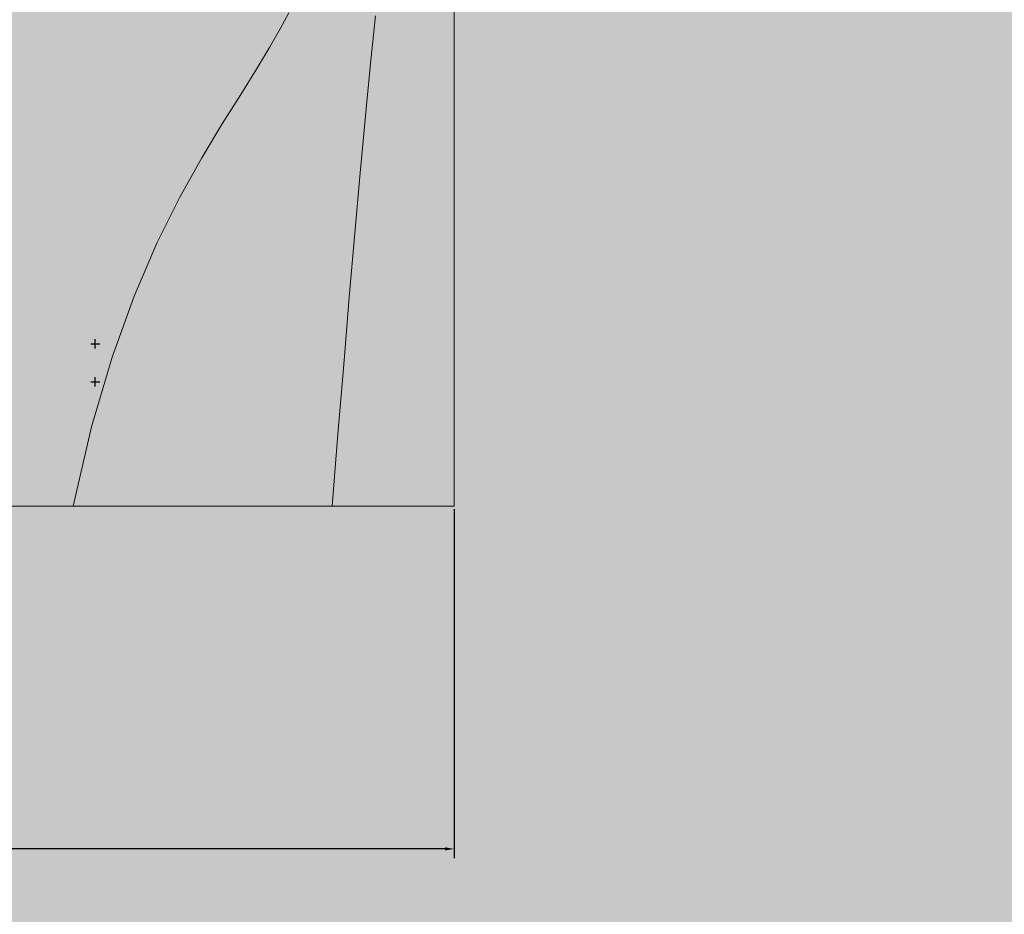
# Model space of a CAD drawing. Units: inches. Extents: x 3024 to 3952, y 1308 to 1863.
# Tile 16 of 29: x 3411.08 to 3430.42, y 1488.75 to 1506.34. Entities that reach past the tile are written whole.
import ezdxf

# ---------------------------------------------------------------- set-up
doc = ezdxf.new("R2010")
doc.units = ezdxf.units.IN
for name, color, linetype, lineweight in [('A-ANNO-DIMS', 2, 'Continuous', 18), ('A-FLOR-TILE-PATT', 7, 'Continuous', 13), ('A-FURN', 8, 'Continuous', 18), ('A-FURN-PATT', 9, 'Continuous', 13)]:
    doc.layers.add(name, color=color, linetype=linetype, lineweight=lineweight)
doc.layers.add('A-FLOR-PATT', color=254, linetype='Continuous', lineweight=13, true_color=0xfeeab9)
doc.styles.get("Standard").update_dxf_attribs({"font": 'arial.ttf'})
doc.dimstyles.get("Standard").update_dxf_attribs({"dimtxt": 0.18, "dimasz": 0.18, "dimexe": 0.18, "dimexo": 0.0625, "dimgap": 0.09, "dimtad": 0, "dimtih": 1, "dimtoh": 1, "dimdec": 4, "dimzin": 0, "dimdsep": 46, "dimtxsty": 'Standard', "dimcen": 0.09, "dimadec": 0, "dimazin": 0, "dimtfac": 1, "dimtdec": 4, "dimtofl": 0, "dimtmove": 0, "dimatfit": 3, "dimfxl": 1, "dimtolj": 1, "dimtzin": 0, "dimarcsym": 0})

# ---------------------------------------------------------------- blocks, each defined once
blk = doc.blocks.new('Table - Rectangular Woodgrain 60 x 30 in.')
for p, q in [((60, 0), (0, 0)), ((60, -30), (60, 0))]:
    blk.add_line(p, q)
for points in [[(47.1333, -2.0667), (48.3862, -2.1947), (49.7625, -2.3281), (51.2513, -2.4663), (52.8416, -2.6083), (54.5226, -2.7535), (56.2833, -2.9011), (58.1127, -3.0501), (60, -3.2)], [(47.0542, -4.3417), (47.4756, -4.5629), (47.9661, -4.8427), (48.5372, -5.1866), (49.2, -5.6), (49.9676, -6.0844), (50.8594, -6.625), (51.8965, -7.2031), (53.1, -7.8), (54.491, -8.3969), (56.0906, -8.975), (57.9199, -9.5156), (60, -10)]]:
    blk.add_lwpolyline(points)
blk = doc.blocks.new('*D33')
at = {"layer": 'A-ANNO-DIMS', "color": 0, "lineweight": -2, "transparency": 16777216}
for p, q in [((3397.15, 1496.716), (3397.15, 1489.858)), ((3419.618, 1496.716), (3419.618, 1489.858)), ((3397.33, 1490.038), (3408.165, 1490.038)), ((3419.438, 1490.038), (3408.604, 1490.038))]:
    blk.add_line(p, q, dxfattribs=at)
at = {"layer": 'A-ANNO-DIMS', "color": 0, "transparency": 16777216}
for points in [[(3397.33, 1490.068), (3397.33, 1490.008), (3397.15, 1490.038)], [(3419.438, 1490.068), (3419.438, 1490.008), (3419.618, 1490.038)]]:
    blk.add_solid(points, dxfattribs=at)
at = {"layer": 'Defpoints', "color": 0, "transparency": 16777216}
for p in [(3397.15, 1496.778), (3419.618, 1496.778), (3419.618, 1490.038)]:
    blk.add_point(p, dxfattribs=at)
at = {"layer": 'A-ANNO-DIMS', "color": 0, "transparency": 16777216, "insert": (3408.384, 1490.038), "char_height": 0.18, "attachment_point": 5}
blk.add_mtext('\\A1;22', dxfattribs=at)
blk = doc.blocks.new('*D107')
at = {"layer": 'A-ANNO-DIMS', "color": 0, "lineweight": -2, "transparency": 16777216}
for p, q in [((3412.475, 1499.22), (3412.655, 1499.22)), ((3412.565, 1499.13), (3412.565, 1499.31)), ((3412.565, 1435.781), (3412.565, 1459.391)), ((3412.745, 1435.781), (3412.565, 1435.781))]:
    blk.add_line(p, q, dxfattribs=at)
at = {"layer": 'A-ANNO-DIMS', "color": 0, "transparency": 16777216}
blk.add_solid([(3412.595, 1459.391), (3412.535, 1459.391), (3412.565, 1459.571)], dxfattribs=at)
at = {"layer": 'Defpoints', "color": 0, "transparency": 16777216}
for p in [(3412.565, 1499.22), (3412.565, 1459.571)]:
    blk.add_point(p, dxfattribs=at)
at = {"layer": 'A-ANNO-DIMS', "color": 0, "transparency": 16777216, "insert": (3413.226, 1435.781), "char_height": 0.18, "attachment_point": 5}
blk.add_mtext('\\A1;R39.65', dxfattribs=at)
blk = doc.blocks.new('*D108')
at = {"layer": 'A-ANNO-DIMS', "color": 0, "lineweight": -2, "transparency": 16777216}
for p, q in [((3412.475, 1499.966), (3412.655, 1499.966)), ((3412.565, 1499.876), (3412.565, 1500.056)), ((3412.565, 1441.651), (3412.565, 1463.339)), ((3412.745, 1441.651), (3412.565, 1441.651))]:
    blk.add_line(p, q, dxfattribs=at)
at = {"layer": 'A-ANNO-DIMS', "color": 0, "transparency": 16777216}
blk.add_solid([(3412.595, 1463.339), (3412.535, 1463.339), (3412.565, 1463.519)], dxfattribs=at)
at = {"layer": 'Defpoints', "color": 0, "transparency": 16777216}
for p in [(3412.565, 1499.966), (3412.565, 1463.519)]:
    blk.add_point(p, dxfattribs=at)
at = {"layer": 'A-ANNO-DIMS', "color": 0, "transparency": 16777216, "insert": (3413.226, 1441.651), "char_height": 0.18, "attachment_point": 5}
blk.add_mtext('\\A1;R36.45', dxfattribs=at)

msp = doc.modelspace()

# ---------------------------------------------------------------- hatches: boundary and pattern name
at = {"layer": 'A-FLOR-PATT', "transparency": 33554528}
h = msp.add_hatch(color=256, dxfattribs=at)
h.dxf.hatch_style = 1
h.paths.add_polyline_path([(3460.764, 1688.6064), (3412.764, 1688.6064), (3412.764, 1694.6064), (3460.764, 1694.6064), (3460.764, 1778.6064), (3406.764, 1778.6064), (3406.764, 1759.9514), (3318.2981, 1759.9514), (3318.2981, 1658.6064), (3322.5356, 1658.6064), (3322.5356, 1652.6064), (3292.764, 1652.6064), (3292.764, 1778.6064), (3106.764, 1778.6064), (3106.764, 1628.6064), (3172.764, 1628.6064), (3172.764, 1532.6064), (3166.764, 1532.6064), (3166.764, 1628.6064), (3106.764, 1628.6064), (3106.764, 1356.8452), (3202.812, 1356.8452), (3202.812, 1354.2534), (3202.812, 1353.8388), (3202.812, 1351.1212), (3202.812, 1347.8452), (3277.764, 1347.8452), (3277.764, 1353.8452), (3277.764, 1356.8452), (3277.764, 1442.6064), (3460.764, 1442.6064)])
h.paths.add_polyline_path([(3216.238, 1527.2064), (3216.238, 1491.2064), (3214.663, 1491.2064), (3214.663, 1491.2409, -0.3966224), (3180.243, 1526.6064), (3163.0285, 1526.6064), (3163.0285, 1531.1064), (3161.716, 1531.1064), (3161.716, 1561.1064), (3163.0285, 1561.1064), (3163.0285, 1531.1064), (3163.0285, 1526.6064), (3180.243, 1526.6064, 0.3966224), (3214.663, 1491.2409), (3214.663, 1527.2064)], flags=16)
h.paths.add_polyline_path([(3227.364, 1649.8972), (3191.364, 1649.8972), (3191.364, 1651.4722), (3227.364, 1651.4722)], flags=16)
h.paths.add_polyline_path([(3323.1172, 1606.7362), (3323.8545, 1606.8514), (3323.8545, 1594.8241), (3323.1172, 1594.9393)], flags=16)
h.paths.add_polyline_path([(3324.2232, 1606.909), (3330.1216, 1607.8307), (3330.1216, 1614.1093), (3339.3495, 1614.1093), (3340.2711, 1620.0078), (3352.4136, 1620.0078), (3353.3353, 1614.1093), (3359.9941, 1614.1093), (3360.9157, 1620.0078), (3373.0582, 1620.0078), (3373.9799, 1614.1093), (3383.2077, 1614.1093), (3383.2077, 1607.8307), (3389.1062, 1606.909), (3389.1062, 1594.7665), (3383.2077, 1593.8449), (3383.2077, 1587.5663), (3373.9799, 1587.5663), (3373.0583, 1581.6678), (3360.9157, 1581.6678), (3359.9941, 1587.5663), (3353.3353, 1587.5663), (3352.4136, 1581.6678), (3340.2711, 1581.6678), (3339.3495, 1587.5663), (3330.1216, 1587.5663), (3330.1216, 1593.8449), (3324.2232, 1594.7665)], flags=16)
h.paths.add_polyline_path([(3236.1584, 1693.1064), (3236.1584, 1723.1064), (3237.4709, 1723.1064), (3237.4709, 1693.1064)], flags=16)
h.paths.add_polyline_path([(3373.2158, 1600.6847), (3373.7965, 1600.7303), (3374.3268, 1600.7874), (3374.8132, 1600.8531), (3375.2621, 1600.9247), (3375.6801, 1600.9991), (3376.0736, 1601.0735), (3376.6855, 1601.19), (3377.366, 1601.3023), (3378.0667, 1601.3814), (3378.8026, 1601.4123), (3379.5865, 1601.3839), (3380.4537, 1601.2948), (3381.301, 1601.1717), (3382.0317, 1601.0433), (3382.4398, 1600.9607), (3382.6252, 1600.9201), (3382.919, 1600.8507), (3382.9044, 1600.8531), (3382.842, 1600.8678), (3382.7541, 1600.8896), (3382.6252, 1600.9201), (3382.4398, 1600.9607), (3382.1868, 1601.0119), (3381.8738, 1601.0711), (3381.5125, 1601.1346), (3381.1149, 1601.1988), (3380.6928, 1601.2601), (3380.2581, 1601.3149), (3379.8226, 1601.3597), (3379.3984, 1601.3908), (3378.9944, 1601.4054), (3378.6092, 1601.4042), (3378.2384, 1601.3886), (3377.8777, 1601.36), (3377.5227, 1601.32), (3377.1691, 1601.2698), (3376.8127, 1601.211), (3376.4491, 1601.145), (3376.0736, 1601.0735), (3375.4177, 1600.9494), (3374.5542, 1600.8119), (3373.5044, 1600.6988)], flags=0)
h.paths.add_polyline_path([(3380.0253, 1596.7351), (3380.499, 1596.6659), (3380.9706, 1596.6119), (3381.4375, 1596.5791), (3381.8971, 1596.5736), (3382.5886, 1596.6167), (3382.7848, 1596.6692), (3382.1465, 1596.5706), (3381.236, 1596.5815), (3380.3199, 1596.6865)], flags=0)
h.paths.add_polyline_path([(3369.6414, 1603.9617), (3370.1589, 1604.0021), (3370.6218, 1604.0539), (3371.0335, 1604.1173), (3371.3978, 1604.1921), (3371.7181, 1604.2785), (3371.9984, 1604.3761), (3372.2441, 1604.483), (3372.4611, 1604.5972), (3372.655, 1604.7163), (3372.8317, 1604.8384), (3372.9968, 1604.9611), (3373.3703, 1605.2455), (3373.8426, 1605.5328), (3374.4624, 1605.7539), (3375.1058, 1605.8302), (3375.7221, 1605.8261), (3376.4109, 1605.76), (3377.1534, 1605.6376), (3377.8945, 1605.473), (3378.1382, 1605.409), (3377.7394, 1605.5074), (3377.3509, 1605.5937), (3376.9704, 1605.6677), (3376.5999, 1605.7288), (3376.2417, 1605.7762), (3375.8979, 1605.8092), (3375.5707, 1605.8271), (3375.2621, 1605.8291), (3374.9745, 1605.8146), (3374.7092, 1605.7832), (3374.4647, 1605.7359), (3374.239, 1605.6742), (3374.0298, 1605.5996), (3373.835, 1605.5134), (3373.6525, 1605.4171), (3373.4801, 1605.3123), (3373.3156, 1605.2002), (3373.1562, 1605.0825), (3372.7603, 1604.781), (3372.236, 1604.4588), (3371.5738, 1604.2283), (3370.8493, 1604.0794), (3369.9262, 1603.976)], flags=0)
h.paths.add_polyline_path([(3366.7533, 1606.5832), (3367.1713, 1606.5519), (3367.5378, 1606.5374), (3367.8568, 1606.5394), (3368.1325, 1606.5573), (3368.3694, 1606.5903), (3368.5717, 1606.6377), (3368.7438, 1606.6988), (3368.89, 1606.7728), (3369.0146, 1606.8591), (3369.121, 1606.9568), (3369.2094, 1607.0646), (3369.2792, 1607.181), (3369.3295, 1607.3046), (3369.3596, 1607.4339), (3369.3688, 1607.5676), (3369.3565, 1607.7042), (3369.3218, 1607.8422), (3369.2649, 1607.9804), (3369.1893, 1608.1187), (3369.0993, 1608.2569), (3368.9992, 1608.3952), (3368.8934, 1608.5334), (3368.7861, 1608.6717), (3368.6817, 1608.8099), (3368.4212, 1609.1804), (3368.2685, 1609.7106), (3368.4883, 1610.1814), (3369.0537, 1610.4604), (3369.6717, 1610.5097), (3370.2812, 1610.3612), (3370.4805, 1610.2968), (3370.1882, 1610.3839), (3369.9284, 1610.4472), (3369.6905, 1610.4842), (3369.4662, 1610.4933), (3369.2555, 1610.4765), (3369.0608, 1610.4367), (3368.884, 1610.3767), (3368.7274, 1610.2994), (3368.5931, 1610.2077), (3368.4833, 1610.1045), (3368.4002, 1609.9927), (3368.3451, 1609.8747), (3368.3166, 1609.7517), (3368.3127, 1609.6244), (3368.331, 1609.4935), (3368.3696, 1609.3597), (3368.4261, 1609.2237), (3368.4985, 1609.0863), (3368.5845, 1608.9482), (3368.6817, 1608.8099), (3368.7861, 1608.6717), (3368.8934, 1608.5334), (3368.9992, 1608.3952), (3369.0993, 1608.2569), (3369.3398, 1607.8876), (3369.3941, 1607.2896), (3368.9774, 1606.7817), (3368.3928, 1606.5742), (3367.7162, 1606.5303), (3367.0044, 1606.5585)], flags=0)
h.paths.add_polyline_path([(3362.1859, 1610.2589), (3362.5478, 1610.2845), (3362.8348, 1610.3275), (3363.0585, 1610.3863), (3363.2303, 1610.4595), (3363.3619, 1610.5457), (3363.463, 1610.6432), (3363.5376, 1610.7502), (3363.5876, 1610.8643), (3363.6153, 1610.9834), (3363.6229, 1611.1055), (3363.6125, 1611.2283), (3363.5861, 1611.3496), (3363.5462, 1611.4673), (3363.4949, 1611.5797), (3363.4358, 1611.6871), (3363.3723, 1611.7902), (3363.3081, 1611.8897), (3363.2468, 1611.9863), (3363.192, 1612.0808), (3363.0258, 1612.4261), (3363.3371, 1612.8672), (3363.9008, 1612.9782), (3364.4822, 1612.9641), (3365.1098, 1612.9074), (3365.328, 1612.8805), (3364.9615, 1612.9208), (3364.6426, 1612.9496), (3364.3668, 1612.9669), (3364.1299, 1612.9726), (3363.9276, 1612.9669), (3363.7555, 1612.9496), (3363.6093, 1612.9208), (3363.4848, 1612.8805), (3363.3782, 1612.8289), (3363.2889, 1612.7672), (3363.2169, 1612.6969), (3363.1622, 1612.6193), (3363.1247, 1612.5361), (3363.1046, 1612.4484), (3363.1017, 1612.358), (3363.1161, 1612.266), (3363.1472, 1612.1738), (3363.192, 1612.0808), (3363.2468, 1611.9863), (3363.3081, 1611.8897), (3363.3723, 1611.7902), (3363.4358, 1611.6871), (3363.6363, 1611.323), (3363.5979, 1610.7003), (3363.0863, 1610.3651), (3362.3983, 1610.2622)], flags=0)
h.paths.add_polyline_path([(3352.356, 1581.2991), (3352.2408, 1580.5618), (3340.4439, 1580.5618), (3340.3287, 1581.2991)], flags=16)
h.paths.add_polyline_path([(3340.4439, 1621.1137), (3352.2408, 1621.1137), (3352.356, 1620.3764), (3340.3287, 1620.3764)], flags=16)
h.paths.add_polyline_path([(3278.4282, 1504.7424), (3290.3831, 1504.7424), (3290.3831, 1502.7499), (3291.0473, 1502.7499), (3291.0473, 1494.7799), (3290.3831, 1494.7799), (3290.3831, 1494.1158), (3291.0473, 1494.1158), (3291.0473, 1486.1458), (3290.3831, 1486.1458), (3290.3831, 1484.1533), (3291.0473, 1484.1533), (3291.0473, 1483.4892, -0.0909091), (3291.0473, 1468.8776), (3291.0473, 1468.2135), (3290.3831, 1468.2135), (3290.3831, 1464.8926), (3278.4282, 1464.8926), (3278.4282, 1472.8626), (3277.764, 1473.5268), (3277.764, 1478.84), (3278.4282, 1479.5042)], flags=16)
h.paths.add_polyline_path([(3278.7603, 1504.4103), (3290.051, 1504.4103), (3290.051, 1465.2247), (3278.7603, 1465.2247)], flags=0)
h.paths.add_polyline_path([(3123.904, 1600.7821), (3117.9039, 1602.7821), (3117.9039, 1599.7821), (3119.4039, 1599.7821), (3119.4039, 1596.7821), (3118.4039, 1596.7821), (3118.4039, 1598.7821), (3117.9039, 1598.7821), (3117.9039, 1596.2821), (3109.9039, 1596.2821), (3109.9039, 1617.2821), (3117.9039, 1617.2821), (3117.9039, 1610.7821), (3123.9038, 1612.7821, -0.7025712), (3137.9039, 1606.7822, -0.7025621)], flags=16)
h.paths.add_polyline_path([(3123.9039, 1602.7822), (3123.9039, 1610.7822, -0.7345333), (3136.9039, 1606.7822, -0.7345297)], flags=0)
h.paths.add_polyline_path([(3177.972, 1689.6473), (3109.2405, 1689.6473), (3109.2405, 1741.1959), (3177.972, 1741.1959)], flags=16)
h.paths.add_polyline_path([(3373.0006, 1581.2991), (3372.8854, 1580.5618), (3361.0885, 1580.5618), (3360.9733, 1581.2991)], flags=16)
h.paths.add_polyline_path([(3361.0885, 1621.1137), (3372.8854, 1621.1137), (3373.0006, 1620.3764), (3360.9733, 1620.3764)], flags=16)
h.paths.add_polyline_path([(3116.9039, 1598.2821, -0.4142136), (3116.1539, 1597.2821), (3111.9039, 1597.2821, -0.4142136), (3110.9039, 1598.0321), (3110.9039, 1615.2821, -0.4142136), (3111.6539, 1616.2821), (3115.9039, 1616.2821, -0.4142136), (3116.9039, 1615.5321)], flags=0)
h.paths.add_polyline_path([(3121.6122, 1728.1369), (3121.6122, 1696.5205), (3110.2715, 1696.5205), (3110.2715, 1714.3906), (3121.6122, 1714.3906), (3121.6122, 1716.4526), (3110.2715, 1716.4526), (3110.2715, 1734.3228), (3123.3304, 1734.3228), (3123.3304, 1729.8552), (3134.6711, 1741.1959), (3134.6711, 1728.1369)], flags=0)
h.paths.add_polyline_path([(3389.4748, 1606.8514), (3390.2122, 1606.7362), (3390.2122, 1594.9393), (3389.4748, 1594.8241)], flags=16)
h.paths.add_polyline_path([(3257.6842, 1762.8281), (3259.6842, 1768.8281), (3256.6842, 1768.8281), (3256.6842, 1767.3281), (3253.6842, 1767.3281), (3253.6842, 1768.3281), (3255.6842, 1768.3281), (3255.6842, 1768.8281), (3253.1842, 1768.8281), (3253.1842, 1776.8281), (3274.1842, 1776.8281), (3274.1842, 1768.8281), (3267.6842, 1768.8281), (3269.6842, 1762.8282, -0.7025712), (3263.6843, 1748.8282, -0.7025621)], flags=16)
h.paths.add_polyline_path([(3259.6842, 1762.8281), (3267.6843, 1762.8281, -0.7345333), (3263.6842, 1749.8282, -0.7345297)], flags=0)
h.paths.add_polyline_path([(3411.264, 1715.6064), (3411.264, 1716.9189), (3441.264, 1716.9189), (3441.264, 1715.6064)], flags=16)
h.paths.add_polyline_path([(3178.3806, 1449.1876), (3178.3806, 1397.639), (3109.6491, 1397.639), (3109.6491, 1449.1876)], flags=16)
h.paths.add_polyline_path([(3397.1501, 1541.7146), (3419.6183, 1541.7146), (3419.6183, 1496.7783), (3397.1501, 1496.7783)], flags=16)
h.paths.add_polyline_path([(3254.1842, 1770.5781), (3254.1842, 1774.8281, -0.4142136), (3254.9342, 1775.8281), (3272.1842, 1775.8281, -0.4142136), (3273.1842, 1775.0781), (3273.1842, 1770.8281, -0.4142136), (3272.4342, 1769.8281), (3255.1842, 1769.8281, -0.4142136)], flags=0)
h.paths.add_polyline_path([(3403.672, 1500.7601), (3403.6016, 1500.3997), (3403.5328, 1500.0441), (3403.4662, 1499.6867), (3403.4027, 1499.3226), (3403.3464, 1498.9532), (3403.3025, 1498.5811), (3403.2759, 1498.2091), (3403.2714, 1497.8401), (3403.3064, 1497.2813), (3403.3491, 1497.1219), (3403.2689, 1497.6395), (3403.2778, 1498.3719), (3403.3635, 1499.0984), (3403.4889, 1499.8168), (3403.6016, 1500.3997), (3403.672, 1500.7601), (3403.744, 1501.1315), (3403.817, 1501.5205), (3403.891, 1501.9336), (3403.9656, 1502.3769), (3404.0404, 1502.8572), (3404.115, 1503.3786), (3404.2264, 1504.2311), (3404.2571, 1504.5223), (3404.1552, 1503.6598), (3404.0063, 1502.6193), (3403.8604, 1501.7518), (3403.744, 1501.1315)], flags=0)
h.paths.add_polyline_path([(3406.5868, 1505.0416), (3406.6121, 1504.5236), (3406.6492, 1504.0526), (3406.6956, 1503.624), (3406.7491, 1503.2333), (3406.8072, 1502.8759), (3406.8676, 1502.5473), (3406.9281, 1502.243), (3407.0268, 1501.7597), (3407.1416, 1501.1368), (3407.2087, 1500.3904), (3407.1804, 1499.6703), (3407.1078, 1498.9956), (3407.0074, 1498.3199), (3406.8809, 1497.6059), (3406.7403, 1496.9627), (3406.7418, 1496.9824), (3406.7491, 1497.0249), (3406.8229, 1497.3409), (3406.8364, 1497.4025), (3406.878, 1497.6078), (3406.9261, 1497.8614), (3406.9777, 1498.1526), (3407.0298, 1498.4712), (3407.0797, 1498.8068), (3407.1243, 1499.149), (3407.1607, 1499.4874), (3407.1859, 1499.8115), (3407.1978, 1500.1137), (3407.1969, 1500.3962), (3407.1841, 1500.6642), (3407.1609, 1500.9225), (3407.1284, 1501.1761), (3407.0876, 1501.43), (3407.0398, 1501.6891), (3406.9862, 1501.9585), (3406.8832, 1502.4628), (3406.7712, 1503.0713), (3406.6657, 1503.8424), (3406.5924, 1504.7735)], flags=0)
h.paths.add_polyline_path([(3409.2517, 1507.8962), (3409.2752, 1507.4282), (3409.3079, 1507.0076), (3409.3501, 1506.6314), (3409.4015, 1506.2969), (3409.4624, 1506.0009), (3409.5326, 1505.7406), (3409.6119, 1505.5128), (3409.6988, 1505.3131), (3409.7915, 1505.1368), (3409.8883, 1504.9792), (3409.9875, 1504.8356), (3410.0872, 1504.7015), (3410.1859, 1504.572), (3410.4508, 1504.2132), (3410.7205, 1503.6035), (3410.8059, 1502.8824), (3410.7619, 1502.0875), (3410.6122, 1501.2299), (3410.4402, 1500.6169), (3410.2538, 1500.0031), (3410.0536, 1499.3219), (3409.9909, 1499.0812), (3410.1761, 1499.7472), (3410.3596, 1500.3513), (3410.4512, 1500.6561), (3410.5312, 1500.9412), (3410.6013, 1501.226), (3410.6614, 1501.512), (3410.7111, 1501.7964), (3410.7496, 1502.0763), (3410.7764, 1502.3489), (3410.7909, 1502.6114), (3410.7926, 1502.8608), (3410.7808, 1503.0944), (3410.7553, 1503.31), (3410.7169, 1503.5087), (3410.6667, 1503.6921), (3410.6061, 1503.8621), (3410.5361, 1504.0203), (3410.4578, 1504.1686), (3410.3726, 1504.3088), (3410.2815, 1504.4424), (3410.1859, 1504.572), (3410.0872, 1504.7015), (3409.859, 1505.0083), (3409.5943, 1505.5117), (3409.4266, 1506.1336), (3409.324, 1506.8011), (3409.2586, 1507.6407)], flags=0)
h.paths.add_polyline_path([(3411.4914, 1510.5878), (3411.4432, 1510.1586), (3411.4054, 1509.775), (3411.38, 1509.4354), (3411.3681, 1509.1376), (3411.3698, 1508.8784), (3411.3843, 1508.6542), (3411.4112, 1508.4618), (3411.4497, 1508.2974), (3411.4994, 1508.1575), (3411.5595, 1508.0388), (3411.6296, 1507.9375), (3411.7097, 1507.851), (3411.802, 1507.7792), (3411.9096, 1507.7225), (3412.0353, 1507.6817), (3412.1821, 1507.6572), (3412.3528, 1507.6496), (3412.5505, 1507.6597), (3412.778, 1507.6879), (3413.0364, 1507.7341), (3413.3194, 1507.7955), (3413.6188, 1507.8687), (3413.9264, 1507.95), (3414.234, 1508.036), (3414.5333, 1508.1232), (3414.8163, 1508.208), (3415.0747, 1508.287), (3415.3023, 1508.3569), (3415.5007, 1508.4158), (3415.6733, 1508.4617), (3416.1158, 1508.5538), (3416.512, 1508.2591), (3416.716, 1507.6581), (3416.61, 1507.0003), (3416.3052, 1506.3411), (3415.8928, 1505.618), (3415.7339, 1505.3633), (3415.9914, 1505.791), (3416.201, 1506.1583), (3416.3666, 1506.4739), (3416.4925, 1506.7462), (3416.5828, 1506.9838), (3416.6413, 1507.1949), (3416.6725, 1507.3883), (3416.6799, 1507.5705), (3416.6662, 1507.7417), (3416.6339, 1507.9), (3416.5851, 1508.0436), (3416.5223, 1508.1709), (3416.4478, 1508.28), (3416.3639, 1508.3692), (3416.273, 1508.4368), (3416.1765, 1508.4815), (3416.0718, 1508.5047), (3415.9553, 1508.5079), (3415.8237, 1508.493), (3415.6733, 1508.4617), (3415.5007, 1508.4158), (3415.3327, 1508.3659), (3414.6495, 1508.157), (3414.0606, 1507.9855), (3413.4456, 1507.8229), (3412.8838, 1507.701), (3412.5505, 1507.6597), (3412.0748, 1507.6354), (3411.595, 1507.8883), (3411.398, 1508.4429), (3411.3624, 1508.9927), (3411.3854, 1509.5711), (3411.4578, 1510.3071)], flags=0)
h.paths.add_polyline_path([(3135.0797, 1449.1876), (3135.0797, 1436.1286), (3122.0208, 1436.1286), (3122.0208, 1404.5122), (3110.6801, 1404.5122), (3110.6801, 1422.3823), (3122.0208, 1422.3823), (3122.0208, 1424.4443), (3110.6801, 1424.4443), (3110.6801, 1442.3145), (3123.739, 1442.3145), (3123.739, 1437.8469)], flags=0)
h.paths.add_polyline_path([(3416.4944, 1514.2949), (3416.4837, 1513.8511), (3416.4893, 1513.4867), (3416.5102, 1513.1926), (3416.5451, 1512.9593), (3416.5929, 1512.7775), (3416.6524, 1512.6379), (3416.7224, 1512.531), (3416.8017, 1512.4488), (3416.8886, 1512.3882), (3416.9813, 1512.3476), (3417.0781, 1512.3251), (3417.1773, 1512.3189), (3417.277, 1512.3274), (3417.3757, 1512.3488), (3417.4713, 1512.3813), (3417.5627, 1512.4229), (3417.65, 1512.471), (3417.7338, 1512.5225), (3417.8146, 1512.5747), (3417.8931, 1512.6245), (3417.9699, 1512.6691), (3418.2968, 1512.8265), (3418.6505, 1512.4645), (3418.7037, 1511.9342), (3418.6693, 1511.3839), (3418.6076, 1510.8228), (3418.5777, 1510.5927), (3418.6197, 1510.9333), (3418.6525, 1511.2311), (3418.6759, 1511.4903), (3418.6899, 1511.7144), (3418.6946, 1511.9069), (3418.6899, 1512.0713), (3418.6759, 1512.2112), (3418.6525, 1512.33), (3418.6197, 1512.4311), (3418.5778, 1512.5177), (3418.5276, 1512.5903), (3418.4705, 1512.6488), (3418.4075, 1512.6933), (3418.3399, 1512.7237), (3418.2686, 1512.7401), (3418.1951, 1512.7424), (3418.1204, 1512.7307), (3418.0455, 1512.7055), (3417.9792, 1512.6736), (3417.65, 1512.471), (3417.5627, 1512.4229), (3417.4713, 1512.3813), (3417.3757, 1512.3488), (3417.277, 1512.3274), (3416.878, 1512.2936), (3416.5757, 1512.7549), (3416.492, 1513.3145), (3416.4808, 1514.0384)], flags=0)
h.paths.add_polyline_path([(3392.8223, 1481.9454), (3396.7707, 1481.9454), (3396.7707, 1480.9201), (3428.3585, 1480.9201), (3428.3585, 1481.9454), (3432.3069, 1481.9454), (3432.3069, 1464.8354, -0.266667), (3392.8223, 1464.8354)], flags=16)
h.paths.add_polyline_path([(3431.203, 1547.5428), (3450.8613, 1547.5428, -0.1904762), (3450.8614, 1484.031), (3431.203, 1484.031), (3431.203, 1488.5675), (3432.3809, 1488.5675), (3432.3809, 1543.0062), (3431.203, 1543.0062)], flags=16)
h.paths.add_polyline_path([(3451.9233, 1524.86, -0.0496282), (3451.9233, 1506.7138), (3446.7921, 1506.7138), (3446.7921, 1524.86)], flags=0)
h.paths.add_polyline_path([(3460.764, 1436.6064), (3277.764, 1436.6064), (3277.764, 1356.8452), (3277.764, 1353.8452), (3460.764, 1353.8452)], flags=17)
h.paths.add_polyline_path([(3121.3033, 1577.378), (3153.693, 1577.378), (3153.693, 1586.6752), (3121.3033, 1586.6752)], flags=24)
h.paths.add_polyline_path([(3164.1457, 1464.1276), (3210.4801, 1464.1276), (3210.4801, 1473.4247), (3164.1457, 1473.4247)], flags=24)
h.paths.add_polyline_path([(3343.1909, 1505.8863), (3373.7236, 1505.8863), (3373.7236, 1515.1773), (3343.1909, 1515.1773)], flags=24)
h.paths.add_polyline_path([(3337.6353, 1564.2926), (3370.0189, 1564.2926), (3370.0189, 1573.5836), (3337.6353, 1573.5836)], flags=24)
h.paths.add_polyline_path([(3419.204, 1753.8578), (3453.3997, 1753.8578), (3453.3997, 1762.9956), (3419.204, 1762.9956)], flags=24)
h.paths.add_polyline_path([(3341.2523, 1701.0246), (3381.0761, 1701.0246), (3381.0761, 1710.3156), (3341.2523, 1710.3156)], flags=24)
h.paths.add_polyline_path([(3245.8895, 1726.2997), (3278.2793, 1726.2997), (3278.2793, 1735.5968), (3245.8895, 1735.5968)], flags=24)
h.paths.add_polyline_path([(3128.8045, 1668.6736), (3175.1389, 1668.6736), (3175.1389, 1677.9707), (3128.8045, 1677.9707)], flags=24)
h.paths.add_polyline_path([(3345.9997, 1396.0062), (3389.09, 1396.0062), (3389.09, 1405.3033), (3345.9997, 1405.3033)], flags=24)
at = {"layer": 'A-FLOR-TILE-PATT', "transparency": 33554569}
h = msp.add_hatch(dxfattribs=at)
h.set_pattern_fill('ANGLE', color=256, scale=2)
h.set_pattern_definition([(0, (0, 0), (0, 13.97), [10.16, -3.81]), (90, (0, 0), (-13.97, 9e-16), [10.16, -3.81])])
h.paths.add_polyline_path([(3292.764, 1778.6064), (3232.764, 1778.6064), (3232.764, 1694.6064), (3236.1584, 1694.6064), (3236.1584, 1723.1064), (3237.4709, 1723.1064), (3237.4709, 1723.0777, -0.3870039), (3266.1209, 1694.6064), (3292.764, 1694.6064)])
h.paths.add_polyline_path([(3263.6843, 1748.8282, -0.7025621), (3257.6842, 1762.8281), (3259.6842, 1768.8281), (3256.6842, 1768.8281), (3256.6842, 1767.3281), (3253.6842, 1767.3281), (3253.6842, 1768.3281), (3255.6842, 1768.3281), (3255.6842, 1768.8281), (3253.1842, 1768.8281), (3253.1842, 1776.8281), (3274.1842, 1776.8281), (3274.1842, 1768.8281), (3267.6842, 1768.8281), (3269.6842, 1762.8282, -0.7025712)], flags=16)
h.paths.add_polyline_path([(3263.6842, 1749.8282, -0.7345297), (3259.6842, 1762.8281), (3267.6843, 1762.8281, -0.7345333)], flags=0)
h.paths.add_polyline_path([(3255.1842, 1769.8281, -0.4142136), (3254.1842, 1770.5781), (3254.1842, 1774.8281, -0.4142136), (3254.9342, 1775.8281), (3272.1842, 1775.8281, -0.4142136), (3273.1842, 1775.0781), (3273.1842, 1770.8281, -0.4142136), (3272.4342, 1769.8281)], flags=0)
h.paths.add_polyline_path([(3460.764, 1436.6064), (3277.764, 1436.6064), (3277.764, 1356.8452), (3277.764, 1353.8452), (3460.764, 1353.8452)])
h.paths.add_polyline_path([(3166.764, 1628.6064), (3106.764, 1628.6064), (3106.764, 1532.6064), (3133.066, 1532.6064, -0.3870039), (3161.716, 1561.0777), (3161.716, 1561.1064), (3163.0285, 1561.1064), (3163.0285, 1532.6064), (3166.764, 1532.6064)])
h.paths.add_polyline_path([(3123.904, 1600.7821), (3117.9039, 1602.7821), (3117.9039, 1599.7821), (3119.4039, 1599.7821), (3119.4039, 1596.7821), (3118.4039, 1596.7821), (3118.4039, 1598.7821), (3117.9039, 1598.7821), (3117.9039, 1596.2821), (3109.9039, 1596.2821), (3109.9039, 1617.2821), (3117.9039, 1617.2821), (3117.9039, 1610.7821), (3123.9038, 1612.7821, -0.7025712), (3137.9039, 1606.7822, -0.7025621)], flags=16)
h.paths.add_polyline_path([(3123.9039, 1602.7822), (3123.9039, 1610.7822, -0.7345333), (3136.9039, 1606.7822, -0.7345297)], flags=0)
h.paths.add_polyline_path([(3116.1539, 1597.2821), (3111.9039, 1597.2821, -0.4142136), (3110.9039, 1598.0321), (3110.9039, 1615.2821, -0.4142136), (3111.6539, 1616.2821), (3115.9039, 1616.2821, -0.4142136), (3116.9039, 1615.5321), (3116.9039, 1598.2821, -0.4142136)], flags=0)
h.paths.add_polyline_path([(3245.8895, 1726.2997), (3278.2793, 1726.2997), (3278.2793, 1735.5968), (3245.8895, 1735.5968)], flags=24)
h.paths.add_polyline_path([(3345.9997, 1396.0062), (3389.09, 1396.0062), (3389.09, 1405.3033), (3345.9997, 1405.3033)], flags=24)
h.paths.add_polyline_path([(3121.3033, 1577.378), (3153.693, 1577.378), (3153.693, 1586.6752), (3121.3033, 1586.6752)], flags=24)
at = {"layer": 'A-FURN-PATT', "transparency": 33554600}
h = msp.add_hatch(color=256, dxfattribs=at)
h.dxf.hatch_style = 1
h.paths.add_polyline_path([(3417.3334, 1524.2182), (3417.4417, 1525.8535), (3417.5429, 1527.6959), (3417.6336, 1529.794), (3417.7102, 1532.1964), (3417.7693, 1534.9516), (3417.8074, 1538.1081), (3417.8209, 1541.7146), (3412.7281, 1541.7146), (3412.8136, 1536.7897), (3412.8505, 1532.7734), (3412.8466, 1529.5424), (3412.8092, 1526.9731), (3412.7461, 1524.942), (3412.6649, 1523.3259), (3412.5731, 1522.0011), (3412.4784, 1520.8443), (3412.3871, 1519.7527), (3412.2998, 1518.707), (3412.216, 1517.7088), (3412.1351, 1516.7594), (3412.0566, 1515.8603), (3411.9799, 1515.013), (3411.9043, 1514.219), (3411.8293, 1513.4797), (3411.7548, 1512.7959), (3411.6819, 1512.1667), (3411.6125, 1511.5901), (3411.5485, 1511.0643), (3411.4914, 1510.5878), (3411.4432, 1510.1586), (3411.4054, 1509.775), (3411.38, 1509.4354), (3411.3681, 1509.1376), (3411.3698, 1508.8784), (3411.3843, 1508.6542), (3411.4112, 1508.4618), (3411.4497, 1508.2974), (3411.4994, 1508.1575), (3411.5595, 1508.0388), (3411.6296, 1507.9375), (3411.7097, 1507.851), (3411.802, 1507.7792), (3411.9096, 1507.7225), (3412.0353, 1507.6817), (3412.1821, 1507.6572), (3412.3528, 1507.6496), (3412.5505, 1507.6597), (3412.778, 1507.6879), (3413.0364, 1507.7341), (3413.3194, 1507.7955), (3413.6188, 1507.8687), (3413.9264, 1507.95), (3414.234, 1508.036), (3414.5333, 1508.1232), (3414.8163, 1508.208), (3415.0747, 1508.287), (3415.4508, 1508.4025), (3415.8572, 1508.5106), (3416.186, 1508.5015), (3416.4107, 1508.3344), (3416.5614, 1508.1136), (3416.6596, 1507.8241), (3416.6872, 1507.4795), (3416.6413, 1507.1949), (3416.5828, 1506.9838), (3416.4925, 1506.7462), (3416.3666, 1506.4739), (3416.201, 1506.1583), (3415.9914, 1505.791), (3415.7339, 1505.3633), (3415.4242, 1504.8669), (3415.0615, 1504.292), (3414.6566, 1503.6241), (3414.2236, 1502.8473), (3413.7766, 1501.946), (3413.3295, 1500.9042), (3412.8966, 1499.7062), (3412.4917, 1498.3362), (3412.1289, 1496.7783), (3417.2217, 1496.7783), (3417.334, 1498.1918), (3417.4456, 1499.5619), (3417.5561, 1500.8806), (3417.6648, 1502.1395), (3417.7712, 1503.3306), (3417.8747, 1504.4456), (3417.9746, 1505.4763), (3418.0705, 1506.4147), (3418.1617, 1507.2549), (3418.2476, 1508.0019), (3418.3277, 1508.6628), (3418.4013, 1509.245), (3418.4679, 1509.7559), (3418.5269, 1510.2027), (3418.5777, 1510.5927), (3418.6197, 1510.9333), (3418.6525, 1511.2311), (3418.6759, 1511.4903), (3418.6899, 1511.7144), (3418.6946, 1511.9069), (3418.6899, 1512.0713), (3418.6759, 1512.2112), (3418.6525, 1512.33), (3418.6197, 1512.4311), (3418.5778, 1512.5177), (3418.5276, 1512.5903), (3418.4705, 1512.6488), (3418.4075, 1512.6933), (3418.3399, 1512.7237), (3418.2686, 1512.7401), (3418.1951, 1512.7424), (3418.1204, 1512.7307), (3418.0455, 1512.7055), (3417.9699, 1512.6691), (3417.8931, 1512.6245), (3417.8146, 1512.5747), (3417.5633, 1512.4125), (3417.2709, 1512.3131), (3416.9695, 1512.3318), (3416.7549, 1512.4815), (3416.6143, 1512.696), (3416.5451, 1512.9593), (3416.5102, 1513.1926), (3416.4893, 1513.4867), (3416.4837, 1513.8511), (3416.4944, 1514.2949), (3416.5226, 1514.8277), (3416.5691, 1515.4576), (3416.6319, 1516.1871), (3416.7088, 1517.0179), (3416.7973, 1517.9515), (3416.8952, 1518.9891), (3417.0002, 1520.1323), (3417.1097, 1521.3827), (3417.2217, 1522.7416)])
h.paths.add_polyline_path([(3419.6183, 1541.7146), (3417.8209, 1541.7146), (3417.8074, 1538.1081), (3417.7693, 1534.9516), (3417.7102, 1532.1964), (3417.6336, 1529.794), (3417.5429, 1527.6959), (3417.4417, 1525.8535), (3417.3334, 1524.2182), (3417.2217, 1522.7416), (3417.1097, 1521.3827), (3417.0002, 1520.1323), (3416.8952, 1518.9891), (3416.7973, 1517.9515), (3416.7088, 1517.0179), (3416.6319, 1516.1871), (3416.5691, 1515.4576), (3416.5226, 1514.8277), (3416.4944, 1514.2949), (3416.4837, 1513.8511), (3416.4893, 1513.4867), (3416.5102, 1513.1926), (3416.5451, 1512.9593), (3416.5929, 1512.7775), (3416.6524, 1512.6379), (3416.7224, 1512.531), (3416.8017, 1512.4488), (3416.8886, 1512.3882), (3416.9813, 1512.3476), (3417.0781, 1512.3251), (3417.1773, 1512.3189), (3417.277, 1512.3274), (3417.3757, 1512.3488), (3417.4713, 1512.3813), (3417.5627, 1512.4229), (3417.65, 1512.471), (3417.7338, 1512.5225), (3417.9865, 1512.6856), (3418.237, 1512.7699), (3418.4785, 1512.6613), (3418.6304, 1512.4416), (3418.6876, 1512.1519), (3418.6969, 1511.8267), (3418.6759, 1511.4903), (3418.6525, 1511.2311), (3418.6197, 1510.9333), (3418.5777, 1510.5927), (3418.5269, 1510.2027), (3418.4679, 1509.7559), (3418.4013, 1509.245), (3418.3277, 1508.6628), (3418.2476, 1508.0019), (3418.1617, 1507.2549), (3418.0705, 1506.4147), (3417.9746, 1505.4763), (3417.8747, 1504.4456), (3417.7712, 1503.3306), (3417.6648, 1502.1395), (3417.5561, 1500.8806), (3417.4456, 1499.5619), (3417.334, 1498.1918), (3417.2217, 1496.7783), (3419.6183, 1496.7783)])
h.paths.add_polyline_path([(3412.5731, 1522.0011), (3412.6649, 1523.3259), (3412.7461, 1524.942), (3412.8092, 1526.9731), (3412.8466, 1529.5424), (3412.8505, 1532.7734), (3412.8136, 1536.7897), (3412.7281, 1541.7146), (3410.0319, 1541.7146), (3409.9329, 1537.8316), (3409.8579, 1534.5089), (3409.8028, 1531.6816), (3409.7635, 1529.2854), (3409.7359, 1527.2554), (3409.7159, 1525.5271), (3409.6994, 1524.0356), (3409.6824, 1522.7166), (3409.6614, 1521.5137), (3409.6364, 1520.405), (3409.6078, 1519.3771), (3409.5763, 1518.4164), (3409.5425, 1517.5096), (3409.5069, 1516.6432), (3409.4701, 1515.8036), (3409.4327, 1514.9775), (3409.3955, 1514.1549), (3409.3594, 1513.3392), (3409.3256, 1512.5376), (3409.2955, 1511.7571), (3409.2699, 1511.0046), (3409.2501, 1510.2873), (3409.2375, 1509.6121), (3409.233, 1508.986), (3409.2377, 1508.4145), (3409.2517, 1507.8962), (3409.2752, 1507.4282), (3409.3079, 1507.0076), (3409.3501, 1506.6314), (3409.4015, 1506.2969), (3409.4624, 1506.0009), (3409.5326, 1505.7406), (3409.6119, 1505.5128), (3409.6988, 1505.3131), (3409.7915, 1505.1368), (3409.8883, 1504.9792), (3409.9875, 1504.8356), (3410.0872, 1504.7015), (3410.3178, 1504.3987), (3410.5042, 1504.0923), (3410.643, 1503.7787), (3410.7431, 1503.4127), (3410.7808, 1503.0944), (3410.7926, 1502.8608), (3410.7909, 1502.6114), (3410.7764, 1502.3489), (3410.7496, 1502.0763), (3410.7111, 1501.7964), (3410.6614, 1501.512), (3410.6013, 1501.226), (3410.5312, 1500.9412), (3410.4512, 1500.6561), (3410.3596, 1500.3513), (3410.2538, 1500.0031), (3410.1317, 1499.5877), (3409.9909, 1499.0812), (3409.8291, 1498.4601), (3409.6438, 1497.7003), (3409.4327, 1496.7783), (3412.1289, 1496.7783), (3412.4917, 1498.3362), (3412.8966, 1499.7062), (3413.3295, 1500.9042), (3413.7766, 1501.946), (3414.2236, 1502.8473), (3414.6566, 1503.6241), (3415.0615, 1504.292), (3415.4242, 1504.8669), (3415.7339, 1505.3633), (3415.9914, 1505.791), (3416.201, 1506.1583), (3416.3666, 1506.4739), (3416.4925, 1506.7462), (3416.5828, 1506.9838), (3416.6413, 1507.1949), (3416.6725, 1507.3883), (3416.6799, 1507.5705), (3416.6662, 1507.7417), (3416.6339, 1507.9), (3416.5851, 1508.0436), (3416.5223, 1508.1709), (3416.4478, 1508.28), (3416.3639, 1508.3692), (3416.273, 1508.4368), (3416.1765, 1508.4815), (3416.0718, 1508.5047), (3415.9553, 1508.5079), (3415.8237, 1508.493), (3415.6733, 1508.4617), (3415.5007, 1508.4158), (3415.3023, 1508.3569), (3414.8599, 1508.2211), (3414.5333, 1508.1232), (3414.234, 1508.036), (3413.9264, 1507.95), (3413.6188, 1507.8687), (3413.3194, 1507.7955), (3412.8838, 1507.701), (3412.4382, 1507.6458), (3412.0995, 1507.6608), (3411.8501, 1507.7418), (3411.666, 1507.885), (3411.5226, 1508.092), (3411.4241, 1508.3695), (3411.3843, 1508.6542), (3411.3698, 1508.8784), (3411.3681, 1509.1376), (3411.38, 1509.4354), (3411.4054, 1509.775), (3411.4432, 1510.1586), (3411.4914, 1510.5878), (3411.5485, 1511.0643), (3411.6125, 1511.5901), (3411.6819, 1512.1667), (3411.7548, 1512.7959), (3411.8293, 1513.4797), (3411.9043, 1514.219), (3411.9799, 1515.013), (3412.0566, 1515.8603), (3412.1351, 1516.7594), (3412.216, 1517.7088), (3412.2998, 1518.707), (3412.3871, 1519.7527), (3412.4784, 1520.8443)])
h.paths.add_polyline_path([(3409.6614, 1521.5137), (3409.6824, 1522.7166), (3409.6994, 1524.0356), (3409.7159, 1525.5271), (3409.7359, 1527.2554), (3409.7635, 1529.2854), (3409.8028, 1531.6816), (3409.8579, 1534.5089), (3409.9329, 1537.8316), (3410.0319, 1541.7146), (3406.1374, 1541.7146), (3406.3416, 1537.8771), (3406.5076, 1534.4792), (3406.639, 1531.4763), (3406.7397, 1528.8235), (3406.8135, 1526.4762), (3406.8641, 1524.3896), (3406.8955, 1522.5188), (3406.9113, 1520.8193), (3406.915, 1519.2519), (3406.9086, 1517.8009), (3406.8933, 1516.4564), (3406.8708, 1515.2084), (3406.8423, 1514.0471), (3406.8095, 1512.9624), (3406.7738, 1511.9444), (3406.7366, 1510.9832), (3406.6994, 1510.0706), (3406.664, 1509.2052), (3406.6321, 1508.3879), (3406.6055, 1507.6192), (3406.5859, 1506.8996), (3406.5751, 1506.2298), (3406.5748, 1505.6103), (3406.5868, 1505.0416), (3406.6121, 1504.5236), (3406.6492, 1504.0526), (3406.6956, 1503.624), (3406.7491, 1503.2333), (3406.8072, 1502.8759), (3406.8676, 1502.5473), (3406.9281, 1502.243), (3407.0268, 1501.7597), (3407.1147, 1501.2828), (3407.1609, 1500.9225), (3407.1841, 1500.6642), (3407.1969, 1500.3962), (3407.1978, 1500.1137), (3407.1859, 1499.8115), (3407.1607, 1499.4874), (3407.1243, 1499.149), (3407.0797, 1498.8068), (3407.0298, 1498.4712), (3406.9777, 1498.1526), (3406.9261, 1497.8614), (3406.8567, 1497.4956), (3406.7944, 1497.2102), (3406.7609, 1497.0755), (3406.7491, 1497.0249), (3406.7418, 1496.9824), (3406.7381, 1496.9355), (3406.7367, 1496.8717), (3406.7366, 1496.7783), (3409.4327, 1496.7783), (3409.6438, 1497.7003), (3409.8291, 1498.4601), (3409.9909, 1499.0812), (3410.1317, 1499.5877), (3410.2538, 1500.0031), (3410.3596, 1500.3513), (3410.4512, 1500.6561), (3410.5312, 1500.9412), (3410.6013, 1501.226), (3410.6614, 1501.512), (3410.7111, 1501.7964), (3410.7496, 1502.0763), (3410.7764, 1502.3489), (3410.7909, 1502.6114), (3410.7926, 1502.8608), (3410.7808, 1503.0944), (3410.7553, 1503.31), (3410.7169, 1503.5087), (3410.6667, 1503.6921), (3410.6061, 1503.8621), (3410.5361, 1504.0203), (3410.4578, 1504.1686), (3410.3726, 1504.3088), (3410.2815, 1504.4424), (3410.1859, 1504.572), (3410.0109, 1504.8017), (3409.8298, 1505.064), (3409.6475, 1505.4106), (3409.5326, 1505.7406), (3409.4624, 1506.0009), (3409.4015, 1506.2969), (3409.3501, 1506.6314), (3409.3079, 1507.0076), (3409.2752, 1507.4282), (3409.2517, 1507.8962), (3409.2377, 1508.4145), (3409.233, 1508.986), (3409.2375, 1509.6121), (3409.2501, 1510.2873), (3409.2699, 1511.0046), (3409.2955, 1511.7571), (3409.3256, 1512.5376), (3409.3594, 1513.3392), (3409.3955, 1514.1549), (3409.4327, 1514.9775), (3409.4701, 1515.8036), (3409.5069, 1516.6432), (3409.5425, 1517.5096), (3409.5763, 1518.4164), (3409.6078, 1519.3771), (3409.6364, 1520.405)])
h.paths.add_polyline_path([(3406.9113, 1520.8193), (3406.8955, 1522.5188), (3406.8641, 1524.3896), (3406.8135, 1526.4762), (3406.7397, 1528.8235), (3406.639, 1531.4763), (3406.5076, 1534.4792), (3406.3416, 1537.8771), (3406.1374, 1541.7146), (3402.8421, 1541.7146), (3402.9543, 1535.7158), (3403.0659, 1530.9229), (3403.1765, 1527.1726), (3403.2852, 1524.3018), (3403.3916, 1522.1472), (3403.4951, 1520.5454), (3403.595, 1519.3334), (3403.6909, 1518.3478), (3403.7822, 1517.4515), (3403.8687, 1516.6123), (3403.9507, 1515.8241), (3404.0279, 1515.0805), (3404.1004, 1514.3756), (3404.1683, 1513.7032), (3404.2315, 1513.0571), (3404.29, 1512.4311), (3404.3436, 1511.8197), (3404.3914, 1511.2188), (3404.4322, 1510.6249), (3404.4648, 1510.0345), (3404.4879, 1509.4441), (3404.5007, 1508.8503), (3404.5017, 1508.2494), (3404.4897, 1507.6379), (3404.4643, 1507.0142), (3404.4265, 1506.3837), (3404.3783, 1505.7534), (3404.3212, 1505.1306), (3404.2571, 1504.5223), (3404.1879, 1503.936), (3404.115, 1503.3786), (3404.0404, 1502.8572), (3403.9656, 1502.3769), (3403.891, 1501.9336), (3403.817, 1501.5205), (3403.744, 1501.1315), (3403.672, 1500.7601), (3403.6016, 1500.3997), (3403.5328, 1500.0441), (3403.4662, 1499.6867), (3403.4027, 1499.3226), (3403.3464, 1498.9532), (3403.3025, 1498.5811), (3403.2759, 1498.2091), (3403.2714, 1497.8401), (3403.2941, 1497.4768), (3403.3491, 1497.1219), (3403.4412, 1496.7783), (3406.7346, 1496.7783), (3406.7393, 1496.9886), (3406.7787, 1497.147), (3406.8034, 1497.2517), (3406.8364, 1497.4025), (3406.878, 1497.6078), (3406.9261, 1497.8614), (3406.9777, 1498.1526), (3407.0298, 1498.4712), (3407.0797, 1498.8068), (3407.1243, 1499.149), (3407.1607, 1499.4874), (3407.1859, 1499.8115), (3407.1978, 1500.1137), (3407.1969, 1500.3962), (3407.1841, 1500.6642), (3407.1609, 1500.9225), (3407.1284, 1501.1761), (3407.0876, 1501.43), (3407.0398, 1501.6891), (3406.9862, 1501.9585), (3406.8832, 1502.4628), (3406.8072, 1502.8759), (3406.7491, 1503.2333), (3406.6956, 1503.624), (3406.6492, 1504.0526), (3406.6121, 1504.5236), (3406.5868, 1505.0416), (3406.5748, 1505.6103), (3406.5751, 1506.2298), (3406.5859, 1506.8996), (3406.6055, 1507.6192), (3406.6321, 1508.3879), (3406.664, 1509.2052), (3406.6994, 1510.0706), (3406.7366, 1510.9832), (3406.7738, 1511.9444), (3406.8095, 1512.9624), (3406.8423, 1514.0471), (3406.8708, 1515.2084), (3406.8933, 1516.4564), (3406.9086, 1517.8009), (3406.915, 1519.2519)])
h.paths.add_polyline_path([(3403.7822, 1517.4515), (3403.6909, 1518.3478), (3403.595, 1519.3334), (3403.4951, 1520.5454), (3403.3916, 1522.1472), (3403.2852, 1524.3018), (3403.1765, 1527.1726), (3403.0659, 1530.9229), (3402.9543, 1535.7158), (3402.8421, 1541.7146), (3400.7451, 1541.7146), (3400.8571, 1535.2472), (3400.9674, 1529.9544), (3401.0741, 1525.6837), (3401.1757, 1522.2828), (3401.2702, 1519.5992), (3401.3559, 1517.4806), (3401.4311, 1515.7745), (3401.494, 1514.3284), (3401.5433, 1513.0143), (3401.5798, 1511.8008), (3401.6046, 1510.6809), (3401.6188, 1509.6476), (3401.6237, 1508.6939), (3401.6203, 1507.8127), (3401.61, 1506.9971), (3401.5938, 1506.2399), (3401.5729, 1505.5342), (3401.5474, 1504.8723), (3401.518, 1504.2464), (3401.4846, 1503.6491), (3401.4478, 1503.0725), (3401.4078, 1502.509), (3401.3648, 1501.9509), (3401.3192, 1501.3905), (3401.2716, 1500.8219), (3401.2236, 1500.246), (3401.1775, 1499.6652), (3401.1351, 1499.0821), (3401.0986, 1498.4993), (3401.0699, 1497.9194), (3401.0513, 1497.3449), (3401.0446, 1496.7783), (3403.4412, 1496.7783), (3403.3491, 1497.1219), (3403.2941, 1497.4768), (3403.2714, 1497.8401), (3403.2759, 1498.2091), (3403.3025, 1498.5811), (3403.3464, 1498.9532), (3403.4027, 1499.3226), (3403.4662, 1499.6867), (3403.5328, 1500.0441), (3403.6016, 1500.3997), (3403.672, 1500.7601), (3403.744, 1501.1315), (3403.817, 1501.5205), (3403.891, 1501.9336), (3403.9656, 1502.3769), (3404.0404, 1502.8572), (3404.115, 1503.3786), (3404.1879, 1503.936), (3404.2571, 1504.5223), (3404.3212, 1505.1306), (3404.3783, 1505.7534), (3404.4265, 1506.3837), (3404.4643, 1507.0142), (3404.4897, 1507.6379), (3404.5017, 1508.2494), (3404.5007, 1508.8503), (3404.4879, 1509.4441), (3404.4648, 1510.0345), (3404.4322, 1510.6249), (3404.3914, 1511.2188), (3404.3436, 1511.8197), (3404.29, 1512.4311), (3404.2315, 1513.0571), (3404.1683, 1513.7032), (3404.1004, 1514.3756), (3404.0279, 1515.0805), (3403.9507, 1515.8241), (3403.8687, 1516.6123)])
h.paths.add_polyline_path([(3401.3559, 1517.4806), (3401.2702, 1519.5992), (3401.1757, 1522.2828), (3401.0741, 1525.6837), (3400.9674, 1529.9544), (3400.8571, 1535.2472), (3400.7451, 1541.7146), (3398.0489, 1541.7146), (3398.1477, 1537.4556), (3398.2213, 1533.8882), (3398.2727, 1530.9247), (3398.3047, 1528.4771), (3398.3204, 1526.4579), (3398.3227, 1524.7793), (3398.3144, 1523.3534), (3398.2985, 1522.0924), (3398.2775, 1520.9226), (3398.2525, 1519.825), (3398.2239, 1518.7946), (3398.1924, 1517.8266), (3398.1586, 1516.9159), (3398.1229, 1516.0576), (3398.0862, 1515.2468), (3398.0489, 1514.4783), (3398.0117, 1513.7461), (3397.9759, 1513.0393), (3397.9431, 1512.346), (3397.9147, 1511.6541), (3397.8921, 1510.9518), (3397.8768, 1510.2269), (3397.8703, 1509.4674), (3397.8741, 1508.6615), (3397.8906, 1507.7925), (3397.926, 1506.8259), (3397.9878, 1505.7222), (3398.0832, 1504.4425), (3398.2196, 1502.9474), (3398.4042, 1501.1979), (3398.6444, 1499.1546), (3398.9476, 1496.7783), (3401.0446, 1496.7783), (3401.0513, 1497.3449), (3401.0699, 1497.9194), (3401.0986, 1498.4993), (3401.1351, 1499.0821), (3401.1775, 1499.6652), (3401.2236, 1500.246), (3401.2716, 1500.8219), (3401.3192, 1501.3905), (3401.3648, 1501.9509), (3401.4078, 1502.509), (3401.4478, 1503.0725), (3401.4846, 1503.6491), (3401.518, 1504.2464), (3401.5474, 1504.8723), (3401.5729, 1505.5342), (3401.5938, 1506.2399), (3401.61, 1506.9971), (3401.6203, 1507.8127), (3401.6237, 1508.6939), (3401.6188, 1509.6476), (3401.6046, 1510.6809), (3401.5798, 1511.8008), (3401.5433, 1513.0143), (3401.494, 1514.3284), (3401.4311, 1515.7745)])
h.paths.add_polyline_path([(3398.3227, 1524.7793), (3398.3204, 1526.4579), (3398.3047, 1528.4771), (3398.2727, 1530.9247), (3398.2213, 1533.8882), (3398.1477, 1537.4556), (3398.0489, 1541.7146), (3397.1501, 1541.7146), (3397.1501, 1496.7783), (3398.9476, 1496.7783), (3398.6444, 1499.1546), (3398.4042, 1501.1979), (3398.2196, 1502.9474), (3398.0832, 1504.4425), (3397.9878, 1505.7222), (3397.926, 1506.8259), (3397.8906, 1507.7925), (3397.8741, 1508.6615), (3397.8703, 1509.4674), (3397.8768, 1510.2269), (3397.8921, 1510.9518), (3397.9147, 1511.6541), (3397.9431, 1512.346), (3397.9759, 1513.0393), (3398.0117, 1513.7461), (3398.0489, 1514.4783), (3398.0862, 1515.2468), (3398.1229, 1516.0576), (3398.1586, 1516.9159), (3398.1924, 1517.8266), (3398.2239, 1518.7946), (3398.2525, 1519.825), (3398.2775, 1520.9226), (3398.2985, 1522.0924), (3398.3144, 1523.3534)])

# ---------------------------------------------------------------- block references
at = {"layer": 'A-FURN', "xscale": 0.7489384925976489, "yscale": 0.7489384925976489, "zscale": 0.7489384925976489, "rotation": 270}
msp.add_blockref('Table - Rectangular Woodgrain 60 x 30 in.', (3419.6183, 1541.7146), dxfattribs=at)

# ---------------------------------------------------------------- dimensions: what is measured, and where the dimension line sits
at = {"layer": 'A-ANNO-DIMS'}
for center, mpoint, picture, middle in [((3412.5646, 1499.9664), (3412.565, 1463.5192), '*D108', (3413.2257, 1441.6508)), ((3412.5646, 1499.2199), (3412.565, 1459.5708), '*D107', (3413.2257, 1435.7813))]:
    dim = msp.add_radius_dim(center=center, mpoint=mpoint, dimstyle='Standard', override={"dimdec": 2, "dimlfac": 1, "dimrnd": 0, "dimzin": 0, "dimdsep": 46, "dimlunit": 2}, dxfattribs=at)
    dim.commit()
    dim.dimension.update_dxf_attribs({"geometry": picture, "text_midpoint": middle, "dimtype": 164})
dim = msp.add_linear_dim(base=(3419.6183, 1490.0379), p1=(3397.1501, 1496.7783), p2=(3419.6183, 1496.7783), dimstyle='Standard', override={"dimdec": 0, "dimlfac": 1, "dimrnd": 0, "dimzin": 0, "dimdsep": 46, "dimlunit": 2}, dxfattribs=at)
dim.commit()
dim.dimension.update_dxf_attribs({"geometry": '*D33', "text_midpoint": (3408.3842, 1490.0379)})

doc.saveas('drawing.dxf')
